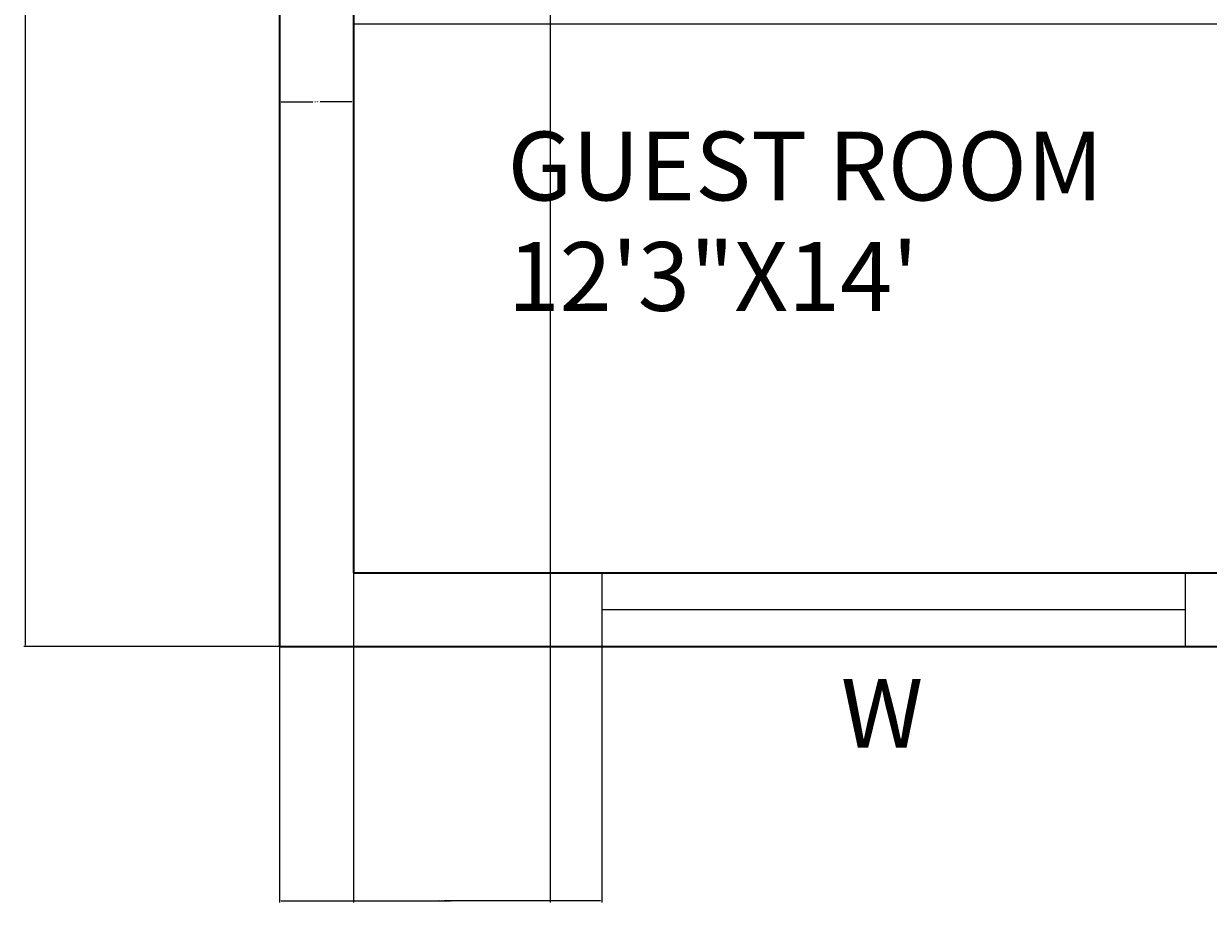
# Model space of a CAD drawing. Units: feet. Extents: x 1654 to 2985, y 1348 to 2230.
# Tile 1 of 53: x 1812 to 1956, y 1534 to 1641. Entities that reach past the tile are written whole.
import ezdxf

# ---------------------------------------------------------------- set-up
doc = ezdxf.new("R2010")
doc.units = ezdxf.units.FT
for name, color, linetype, lineweight in [('A-ANNO-DIMS', 2, 'Continuous', 18), ('A-ANNO-TEXT', 7, 'Continuous', 18), ('A-AREA-IDEN', 7, 'Continuous', 18), ('A-GLAZ', 4, 'Continuous', 18), ('A-WALL', 7, 'Continuous', 35)]:
    doc.layers.add(name, color=color, linetype=linetype, lineweight=lineweight)
doc.styles.get("Standard").update_dxf_attribs({"font": 'arial.ttf'})
doc.dimstyles.get("Standard").update_dxf_attribs({"dimtxt": 0.18, "dimasz": 0.18, "dimexe": 0.18, "dimexo": 0.0625, "dimgap": 0.09, "dimtad": 0, "dimtih": 1, "dimtoh": 1, "dimdec": 4, "dimzin": 0, "dimdsep": 46, "dimtxsty": 'Standard', "dimcen": 0.09, "dimadec": 0, "dimazin": 0, "dimtfac": 1, "dimtdec": 4, "dimtofl": 0, "dimtmove": 0, "dimatfit": 3, "dimfxl": 1, "dimtolj": 1, "dimtzin": 0, "dimarcsym": 0})

# ---------------------------------------------------------------- blocks, each defined once
blk = doc.blocks.new('WIN-GUEST-FRONT')
for p, q in [((0, 9), (0, 0)), ((71.09, 9), (71.09, 0)), ((0, 4.5), (71.09, 4.5))]:
    blk.add_line(p, q)
blk = doc.blocks.new('*D65')
at = {"layer": 'A-ANNO-DIMS', "color": 0, "lineweight": -2, "transparency": 16777216}
for p, q in [((1843.09, 1641.12), (1843.09, 1631.48)), ((1852.09, 1641.12), (1852.09, 1631.48)), ((1843.27, 1631.66), (1847.13, 1631.66)), ((1851.91, 1631.66), (1848.05, 1631.66))]:
    blk.add_line(p, q, dxfattribs=at)
at = {"layer": 'A-ANNO-DIMS', "color": 0, "transparency": 16777216}
for points in [[(1843.27, 1631.69), (1843.27, 1631.63), (1843.09, 1631.66)], [(1851.91, 1631.69), (1851.91, 1631.63), (1852.09, 1631.66)]]:
    blk.add_solid(points, dxfattribs=at)
at = {"layer": 'Defpoints', "color": 0, "transparency": 16777216}
for p in [(1843.09, 1641.19), (1852.09, 1641.19), (1852.09, 1631.66)]:
    blk.add_point(p, dxfattribs=at)
at = {"layer": 'A-ANNO-DIMS', "color": 0, "transparency": 16777216, "insert": (1847.59, 1631.66), "char_height": 0.18, "attachment_point": 5}
blk.add_mtext('\\A1;9 TYP.', dxfattribs=at)
blk = doc.blocks.new('*D77')
at = {"layer": 'A-ANNO-DIMS', "color": 0, "lineweight": -2, "transparency": 16777216}
for p, q in [((1843.03, 2117.25), (1811.91, 2117.25)), ((1812.09, 2117.07), (1812.09, 1841.44)), ((1812.09, 1565.43), (1812.09, 1841.07)), ((1843.03, 1565.25), (1811.91, 1565.25))]:
    blk.add_line(p, q, dxfattribs=at)
at = {"layer": 'A-ANNO-DIMS', "color": 0, "transparency": 16777216}
for points in [[(1812.06, 2117.07), (1812.12, 2117.07), (1812.09, 2117.25)], [(1812.06, 1565.43), (1812.12, 1565.43), (1812.09, 1565.25)]]:
    blk.add_solid(points, dxfattribs=at)
at = {"layer": 'Defpoints', "color": 0, "transparency": 16777216}
for p in [(1812.09, 2117.25), (1843.09, 2117.25), (1843.09, 1565.25)]:
    blk.add_point(p, dxfattribs=at)
at = {"layer": 'A-ANNO-DIMS', "color": 0, "transparency": 16777216, "insert": (1812.09, 1841.25), "char_height": 0.18, "attachment_point": 5}
blk.add_mtext('\\A1;552', dxfattribs=at)
blk = doc.blocks.new('*D89')
at = {"layer": 'A-ANNO-DIMS', "color": 0, "lineweight": -2, "transparency": 16777216}
for p, q in [((1843.09, 1565.19), (1843.09, 1534.07)), ((1882.38, 1565.19), (1882.38, 1534.07)), ((1843.27, 1534.25), (1862.34, 1534.25)), ((1882.2, 1534.25), (1863.13, 1534.25))]:
    blk.add_line(p, q, dxfattribs=at)
at = {"layer": 'A-ANNO-DIMS', "color": 0, "transparency": 16777216}
for points in [[(1843.27, 1534.28), (1843.27, 1534.22), (1843.09, 1534.25)], [(1882.2, 1534.28), (1882.2, 1534.22), (1882.38, 1534.25)]]:
    blk.add_solid(points, dxfattribs=at)
at = {"layer": 'Defpoints', "color": 0, "transparency": 16777216}
for p in [(1843.09, 1565.25), (1882.38, 1565.25), (1882.38, 1534.25)]:
    blk.add_point(p, dxfattribs=at)
at = {"layer": 'A-ANNO-DIMS', "color": 0, "transparency": 16777216, "insert": (1862.74, 1534.25), "char_height": 0.18, "attachment_point": 5}
blk.add_mtext('\\A1;39.29', dxfattribs=at)
blk = doc.blocks.new('*D90')
at = {"layer": 'A-ANNO-DIMS', "color": 0, "lineweight": -2, "transparency": 16777216}
for p, q in [((1852.15, 1641.19), (2242.27, 1641.19)), ((2242.09, 1641.01), (2242.09, 1607.9)), ((2242.09, 1574.43), (2242.09, 1607.54)), ((1852.15, 1574.25), (2242.27, 1574.25))]:
    blk.add_line(p, q, dxfattribs=at)
at = {"layer": 'A-ANNO-DIMS', "color": 0, "transparency": 16777216}
for points in [[(2242.06, 1641.01), (2242.12, 1641.01), (2242.09, 1641.19)], [(2242.06, 1574.43), (2242.12, 1574.43), (2242.09, 1574.25)]]:
    blk.add_solid(points, dxfattribs=at)
at = {"layer": 'Defpoints', "color": 0, "transparency": 16777216}
for p in [(1852.09, 1641.19), (2242.09, 1641.19), (1852.09, 1574.25)]:
    blk.add_point(p, dxfattribs=at)
at = {"layer": 'A-ANNO-DIMS', "color": 0, "transparency": 16777216, "insert": (2242.09, 1607.72), "char_height": 0.18, "attachment_point": 5}
blk.add_mtext('\\A1;66.93', dxfattribs=at)
blk = doc.blocks.new('*D100')
at = {"layer": 'A-ANNO-DIMS', "color": 0, "lineweight": -2, "transparency": 16777216}
for p, q in [((1852.09, 1751.19), (1852.09, 1534.07)), ((1876.09, 1751.19), (1876.09, 1534.07)), ((1852.27, 1534.25), (1863.87, 1534.25)), ((1875.91, 1534.25), (1864.31, 1534.25))]:
    blk.add_line(p, q, dxfattribs=at)
at = {"layer": 'A-ANNO-DIMS', "color": 0, "transparency": 16777216}
for points in [[(1852.27, 1534.28), (1852.27, 1534.22), (1852.09, 1534.25)], [(1875.91, 1534.28), (1875.91, 1534.22), (1876.09, 1534.25)]]:
    blk.add_solid(points, dxfattribs=at)
at = {"layer": 'Defpoints', "color": 0, "transparency": 16777216}
for p in [(1852.09, 1751.25), (1876.09, 1751.25), (1876.09, 1534.25)]:
    blk.add_point(p, dxfattribs=at)
at = {"layer": 'A-ANNO-DIMS', "color": 0, "transparency": 16777216, "insert": (1864.09, 1534.25), "char_height": 0.18, "attachment_point": 5}
blk.add_mtext('\\A1;24', dxfattribs=at)

msp = doc.modelspace()

# ---------------------------------------------------------------- linework, layer by layer
at = {"layer": 'A-WALL'}
for p, q in [((1843.0924, 2117.2549), (1843.0924, 1565.2549)), ((1843.0924, 1742.2549), (1843.0924, 1565.2549)), ((1852.0924, 1742.2549), (1852.0924, 1574.2549)), ((1852.0924, 1574.2549), (1999.0924, 1574.2549)), ((1843.0924, 1565.2549), (2008.0924, 1565.2549))]:
    msp.add_line(p, q, dxfattribs=at)

# ---------------------------------------------------------------- block references
at = {"layer": 'A-GLAZ'}
msp.add_blockref('WIN-GUEST-FRONT', (1882.383, 1565.255), dxfattribs=at)

# ---------------------------------------------------------------- texts
at = {"layer": 'A-ANNO-TEXT'}
msp.add_text('W', height=8.3811, dxfattribs=at).set_placement((1911.5101, 1552.9169))
at = {"layer": 'A-AREA-IDEN'}
for s, p in [('GUEST ROOM', (1870.8823, 1619.6449)), ('12\'3"X14\'', (1870.8823, 1606.1813))]:
    msp.add_text(s, height=8.38114, dxfattribs=at).set_placement(p)

# ---------------------------------------------------------------- dimensions: what is measured, and where the dimension line sits
at = {"layer": 'A-ANNO-DIMS'}
for base, p1, p2, override, picture, middle in [((1812.0924, 2117.2549), (1843.0924, 1565.2549), (1843.0924, 2117.2549), {"dimdec": 0, "dimlfac": 1, "dimrnd": 0, "dimzin": 0, "dimdsep": 46, "dimlunit": 2}, '*D77', (1812.0924, 1841.2549)), ((2242.0924, 1641.187), (1852.0924, 1574.2549), (1852.0924, 1641.187), {"dimdec": 2, "dimlfac": 1, "dimrnd": 0, "dimzin": 0, "dimdsep": 46, "dimlunit": 2}, '*D90', (2242.0924, 1607.721))]:
    dim = msp.add_linear_dim(base=base, p1=p1, p2=p2, angle=90, dimstyle='Standard', override=override, dxfattribs=at)
    dim.commit()
    dim.dimension.update_dxf_attribs({"geometry": picture, "text_midpoint": middle})
for base, p1, p2, override, picture, middle in [((1876.0924, 1534.2549), (1852.0924, 1751.2549), (1876.0924, 1751.2549), {"dimdec": 0, "dimlfac": 1, "dimrnd": 0, "dimzin": 0, "dimdsep": 46, "dimlunit": 2}, '*D100', (1864.0924, 1534.2549)), ((1882.383, 1534.2549), (1843.0924, 1565.2549), (1882.383, 1565.2549), {"dimdec": 2, "dimlfac": 1, "dimrnd": 0, "dimzin": 0, "dimdsep": 46, "dimlunit": 2}, '*D89', (1862.7377, 1534.2549))]:
    dim = msp.add_linear_dim(base=base, p1=p1, p2=p2, dimstyle='Standard', override=override, dxfattribs=at)
    dim.commit()
    dim.dimension.update_dxf_attribs({"geometry": picture, "text_midpoint": middle})
dim = msp.add_linear_dim(base=(1852.0924, 1631.6569), p1=(1843.0924, 1641.187), p2=(1852.0924, 1641.187), text='<> TYP.', dimstyle='Standard', override={"dimdec": 0, "dimlfac": 1, "dimrnd": 0, "dimzin": 0, "dimdsep": 46, "dimlunit": 2}, dxfattribs=at)
dim.commit()
dim.dimension.update_dxf_attribs({"geometry": '*D65', "text_midpoint": (1847.5924, 1631.6569)})

doc.saveas('drawing.dxf')
